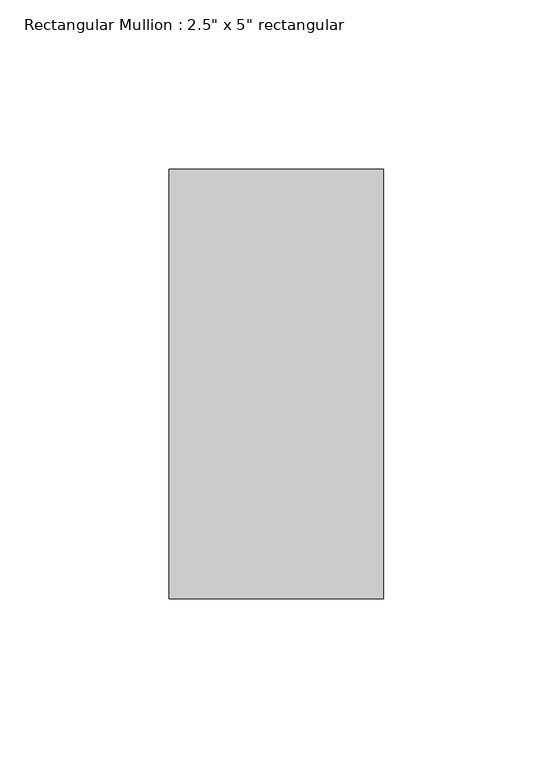
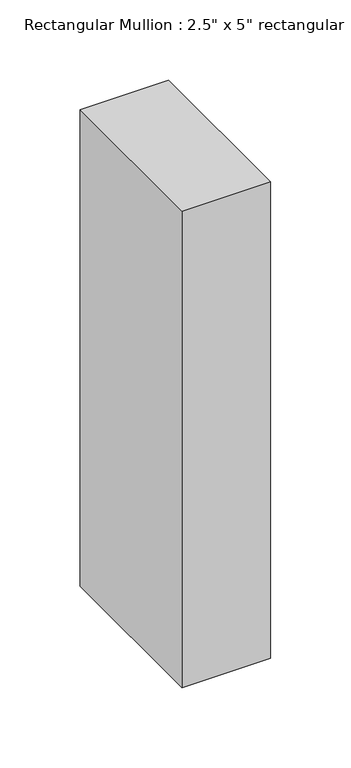
"""IFC4 building model written with IfcOpenShell, lengths in millimetres: member geometry."""

from ifc_helpers import new_model, si_unit, frame, origin, place, context, project, spatial, polyline, outline, extrude, source, transform, mapped, element, save


def member_843225dc(model_context):
    return source(origin(), model_context, "Body", "SweptSolid", [
        extrude(outline(polyline([(0.0, 63.5), (0.0, -63.5), (-63.5, -63.5), (-63.5, 63.5), (0.0, 63.5)])), frame((0.0, 0.0, -361.95), z_axis=(0.0, 0.0, 1.0), x_axis=(1.0, 0.0, 0.0)), (0.0, 0.0, 1.0), 361.95),
    ])


if __name__ == "__main__":
    model = new_model("IFC4")
    model_context = context("Model", 3, world=origin())
    ifc_project = project(units=[si_unit("LENGTHUNIT", "METRE", prefix="MILLI")], contexts=[model_context])
    site = spatial("IfcSite", under=ifc_project)
    building = spatial("IfcBuilding", under=site)
    placement = place(None, origin())
    member_shape = member_843225dc(model_context)
    element("IfcMember", 1, ObjectType="Rectangular Mullion : 2.5\" x 5\" rectangular", at=placement, inside=building, context=model_context, shape_type="MappedRepresentation", body=[
        mapped(member_shape, transform((0.0, 0.0, 0.0), x_axis=(1.0, 0.0, 0.0), y_axis=(0.0, 1.0, 0.0), z_axis=(0.0, 0.0, 1.0))),
    ])
    save(model, "model.ifc")

# Revit data of these elements
# Type "Rectangular Mullion : 2.5\" x 5\" rectangular"
#   built-in parameter 1007304 = 0.416667 (stored number, unit not read)
#   built-in parameter 1007301 = 0.104167 (stored number, unit not read)
#   built-in parameter 1007300 = 0.104167 (stored number, unit not read)
